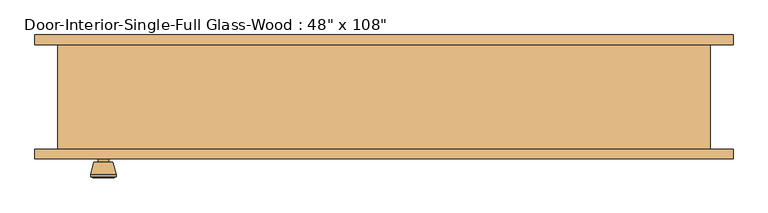
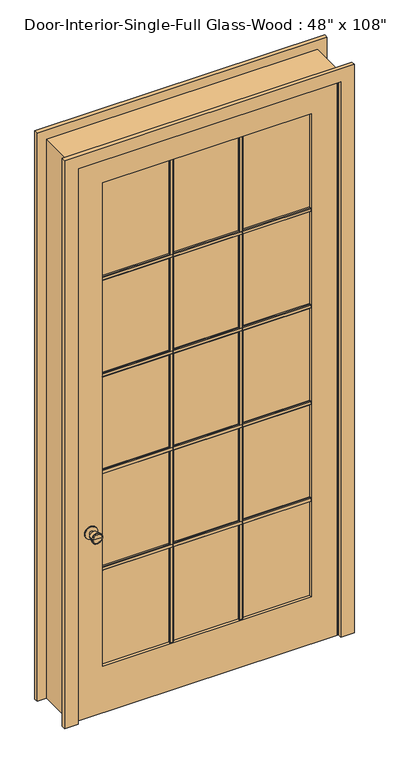
"""IFC4 building model written with IfcOpenShell, lengths in millimetres: door geometry."""

from ifc_helpers import new_model, si_unit, point, frame, frame_2d, origin, place, context, project, spatial, polyline, circle_curve, trimmed, segment, composite_curve, outline, extrude, faceted_brep, source, transform, mapped, element, save
from ifc_brep_helpers import plane_surface, cylinder_surface, revolved_surface, advanced_brep


def door_b9d6288b(model_context):
    return source(origin(), model_context, "Body", "SolidModel", [
        extrude(outline(polyline([(-84.455, 2155.19), (-84.455, 2136.14), (-90.805, 2136.14), (-93.98, 2139.315), (-93.98, 2152.015), (-90.805, 2155.19), (-84.455, 2155.19)])), frame((-488.95, 0.0, 0.0), z_axis=(1.0, 0.0, 0.0), x_axis=(0.0, 1.0, 0.0)), (0.0, 0.0, 1.0), 977.9),
        extrude(outline(polyline([(-84.455, 1676.7175), (-84.455, 1657.6675), (-90.805, 1657.6675), (-93.98, 1660.8425), (-93.98, 1673.5425), (-90.805, 1676.7175), (-84.455, 1676.7175)])), frame((-488.95, 0.0, 0.0), z_axis=(1.0, 0.0, 0.0), x_axis=(0.0, 1.0, 0.0)), (0.0, 0.0, 1.0), 977.9),
        extrude(outline(polyline([(-84.455, 1198.245), (-84.455, 1179.195), (-90.805, 1179.195), (-93.98, 1182.37), (-93.98, 1195.07), (-90.805, 1198.245), (-84.455, 1198.245)])), frame((-488.95, 0.0, 0.0), z_axis=(1.0, 0.0, 0.0), x_axis=(0.0, 1.0, 0.0)), (0.0, 0.0, 1.0), 977.9),
        extrude(outline(polyline([(-84.455, 719.7725), (-84.455, 700.7225), (-90.805, 700.7225), (-93.98, 703.8975), (-93.98, 716.5975), (-90.805, 719.7725), (-84.455, 719.7725)])), frame((-488.95, 0.0, 0.0), z_axis=(1.0, 0.0, 0.0), x_axis=(0.0, 1.0, 0.0)), (0.0, 0.0, 1.0), 977.9),
        extrude(outline(polyline([(153.4583333, -84.455), (172.5083333, -84.455), (172.5083333, -90.805), (169.3333333, -93.98), (156.6333333, -93.98), (153.4583333, -90.805), (153.4583333, -84.455)])), frame((0.0, 0.0, 231.775), z_axis=(0.0, 0.0, 1.0), x_axis=(1.0, 0.0, 0.0)), (0.0, 0.0, 1.0), 2392.3625),
        extrude(outline(polyline([(-172.5083333, -84.455), (-153.4583333, -84.455), (-153.4583333, -90.805), (-156.6333333, -93.98), (-169.3333333, -93.98), (-172.5083333, -90.805), (-172.5083333, -84.455)])), frame((0.0, 0.0, 231.775), z_axis=(0.0, 0.0, 1.0), x_axis=(1.0, 0.0, 0.0)), (0.0, 0.0, 1.0), 2392.3625),
        extrude(outline(polyline([(-77.47, 2155.19), (-71.12, 2155.19), (-67.945, 2152.015), (-67.945, 2139.315), (-71.12, 2136.14), (-77.47, 2136.14), (-77.47, 2155.19)])), frame((-488.95, 0.0, 0.0), z_axis=(1.0, 0.0, 0.0), x_axis=(0.0, 1.0, 0.0)), (0.0, 0.0, 1.0), 977.9),
        extrude(outline(polyline([(-77.47, 1676.7175), (-71.12, 1676.7175), (-67.945, 1673.5425), (-67.945, 1660.8425), (-71.12, 1657.6675), (-77.47, 1657.6675), (-77.47, 1676.7175)])), frame((-488.95, 0.0, 0.0), z_axis=(1.0, 0.0, 0.0), x_axis=(0.0, 1.0, 0.0)), (0.0, 0.0, 1.0), 977.9),
        extrude(outline(polyline([(-77.47, 1198.245), (-71.12, 1198.245), (-67.945, 1195.07), (-67.945, 1182.37), (-71.12, 1179.195), (-77.47, 1179.195), (-77.47, 1198.245)])), frame((-488.95, 0.0, 0.0), z_axis=(1.0, 0.0, 0.0), x_axis=(0.0, 1.0, 0.0)), (0.0, 0.0, 1.0), 977.9),
        extrude(outline(polyline([(-77.47, 719.7725), (-71.12, 719.7725), (-67.945, 716.5975), (-67.945, 703.8975), (-71.12, 700.7225), (-77.47, 700.7225), (-77.47, 719.7725)])), frame((-488.95, 0.0, 0.0), z_axis=(1.0, 0.0, 0.0), x_axis=(0.0, 1.0, 0.0)), (0.0, 0.0, 1.0), 977.9),
        extrude(outline(polyline([(153.4583333, -77.47), (153.4583333, -71.12), (156.6333333, -67.945), (169.3333333, -67.945), (172.5083333, -71.12), (172.5083333, -77.47), (153.4583333, -77.47)])), frame((0.0, 0.0, 231.775), z_axis=(0.0, 0.0, 1.0), x_axis=(1.0, 0.0, 0.0)), (0.0, 0.0, 1.0), 2392.3625),
        extrude(outline(polyline([(-172.5083333, -77.47), (-172.5083333, -71.12), (-169.3333333, -67.945), (-156.6333333, -67.945), (-153.4583333, -71.12), (-153.4583333, -77.47), (-172.5083333, -77.47)])), frame((0.0, 0.0, 231.775), z_axis=(0.0, 0.0, 1.0), x_axis=(1.0, 0.0, 0.0)), (0.0, 0.0, 1.0), 2392.3625),
        advanced_brep(
        [(-546.1, -57.5, 914.4), (-556.1, -57.5, 914.4), (-536.1, -57.5, 914.4), (-525.6241324, -8.5, 914.4), (-566.5758676, -8.5, 914.4), (-546.1, -8.5, 914.4), (-521.1, -10.3278681, 914.4), (-571.1, -10.3278681, 914.4), (-521.1, -13.7915463, 914.4), (-571.1, -13.7915463, 914.4), (-527.463764, -38.5, 914.4), (-564.736236, -38.5, 914.4), (-536.1, -38.5, 914.4), (-556.1, -38.5, 914.4)],
        [
            (0, 1),
            (1, 2, circle_curve(frame((-546.1, -57.5, 914.4), z_axis=(0.0, -1.0, 0.0), x_axis=(-1.0, 0.0, 0.0)), 10.0)),
            (2, 0),
            (2, 1, circle_curve(frame((-546.1, -57.5, 914.4), z_axis=(0.0, -1.0, 0.0), x_axis=(-1.0, 0.0, 0.0)), 10.0)),
            (3, 4, circle_curve(frame((-546.1, -8.5, 914.4), z_axis=(0.0, 1.0, 0.0), x_axis=(-1.0, 0.0, 0.0)), 20.4758676)),
            (4, 5),
            (5, 3),
            (4, 3, circle_curve(frame((-546.1, -8.5, 914.4), z_axis=(0.0, 1.0, 0.0), x_axis=(-1.0, 0.0, 0.0)), 20.4758676)),
            (6, 7, circle_curve(frame((-546.1, -10.3278681, 914.4), z_axis=(0.0, 1.0, 0.0), x_axis=(-1.0, 0.0, 0.0)), 25.0)),
            (7, 4),
            (3, 6),
            (7, 6, circle_curve(frame((-546.1, -10.3278681, 914.4), z_axis=(0.0, 1.0, 0.0), x_axis=(-1.0, 0.0, 0.0)), 25.0)),
            (8, 9, circle_curve(frame((-546.1, -13.7915463, 914.4), z_axis=(0.0, 1.0, 0.0), x_axis=(-1.0, 0.0, 0.0)), 25.0)),
            (9, 7),
            (6, 8),
            (9, 8, circle_curve(frame((-546.1, -13.7915463, 914.4), z_axis=(0.0, 1.0, 0.0), x_axis=(-1.0, 0.0, 0.0)), 25.0)),
            (10, 11, circle_curve(frame((-546.1, -38.5, 914.4), z_axis=(0.0, 1.0, 0.0), x_axis=(-1.0, 0.0, 0.0)), 18.636236)),
            (11, 9),
            (8, 10),
            (11, 10, circle_curve(frame((-546.1, -38.5, 914.4), z_axis=(0.0, 1.0, 0.0), x_axis=(-1.0, 0.0, 0.0)), 18.636236)),
            (12, 13, circle_curve(frame((-546.1, -38.5, 914.4), z_axis=(0.0, 1.0, 0.0), x_axis=(-1.0, 0.0, 0.0)), 10.0)),
            (13, 11),
            (10, 12),
            (13, 12, circle_curve(frame((-546.1, -38.5, 914.4), z_axis=(0.0, 1.0, 0.0), x_axis=(-1.0, 0.0, 0.0)), 10.0)),
            (1, 13),
            (12, 2),
        ],
        [
            plane_surface(frame((-546.1, -57.5, 914.4), z_axis=(0.0, -1.0, 0.0), x_axis=(-1.0, 0.0, 0.0))),
            plane_surface(frame((-546.1, -8.5, 914.4), z_axis=(0.0, 1.0, 0.0), x_axis=(-1.0, 0.0, 0.0))),
            revolved_surface(polyline([(-566.5758676, -8.5, 914.4), (-571.1, -10.3278681, 914.4)]), (-546.1, -57.5, 914.4), (0.0, -1.0, 0.0)),
            cylinder_surface(frame((-546.1, -57.5, 914.4), z_axis=(0.0, -1.0, 0.0), x_axis=(-1.0, 0.0, 0.0)), 25.0),
            revolved_surface(polyline([(-571.1, -13.7915463, 914.4), (-564.736236, -38.5, 914.4)]), (-546.1, -57.5, 914.4), (0.0, -1.0, 0.0)),
            plane_surface(frame((-546.1, -38.5, 914.4), z_axis=(0.0, -1.0, 0.0), x_axis=(-1.0, 0.0, 0.0))),
            cylinder_surface(frame((-546.1, -57.5, 914.4), z_axis=(0.0, -1.0, 0.0), x_axis=(-1.0, 0.0, 0.0)), 10.0),
        ],
        [
            (0, [[1, 2, 3]]),
            (0, [[-3, 4, -1]]),
            (1, [[5, 6, 7]]),
            (1, [[8, -7, -6]]),
            (2, [[9, 10, -5, 11]]),
            (2, [[12, -11, -8, -10]]),
            (3, [[13, 14, -9, 15]]),
            (3, [[16, -15, -12, -14]]),
            (4, [[17, 18, -13, 19]]),
            (4, [[20, -19, -16, -18]]),
            (5, [[21, 22, -17, 23]]),
            (5, [[24, -23, -20, -22]]),
            (6, [[-2, 25, -21, 26]]),
            (6, [[-4, -26, -24, -25]]),
        ],
    ),
        extrude(outline(composite_curve([segment(trimmed(circle_curve(frame_2d((914.4, -546.1)), 30.0), [point((914.4, -576.1))], [point((914.4, -516.1))], False, "CARTESIAN"), True, "CONTINUOUS"), segment(trimmed(circle_curve(frame_2d((914.4, -546.1)), 30.0), [point((914.4, -516.1))], [point((914.4, -576.1))], False, "CARTESIAN"), True, "CONTINUOUS")], self_intersect=False)), frame((0.0, -63.5, 0.0), z_axis=(0.0, 1.0, 0.0), x_axis=(0.0, 0.0, 1.0)), (0.0, 0.0, 1.0), 6.0),
        advanced_brep(
        [(-546.1, -104.425, 914.4), (-536.1, -104.425, 914.4), (-556.1, -104.425, 914.4), (-525.6241324, -153.425, 914.4), (-546.1, -153.425, 914.4), (-566.5758676, -153.425, 914.4), (-521.1, -151.5971319, 914.4), (-571.1, -151.5971319, 914.4), (-521.1, -148.1334537, 914.4), (-571.1, -148.1334537, 914.4), (-527.463764, -123.425, 914.4), (-564.736236, -123.425, 914.4), (-536.1, -123.425, 914.4), (-556.1, -123.425, 914.4)],
        [
            (0, 1),
            (1, 2, circle_curve(frame((-546.1, -104.425, 914.4), z_axis=(0.0, 1.0, 0.0), x_axis=(-1.0, 0.0, 0.0)), 10.0)),
            (2, 0),
            (2, 1, circle_curve(frame((-546.1, -104.425, 914.4), z_axis=(0.0, 1.0, 0.0), x_axis=(-1.0, 0.0, 0.0)), 10.0)),
            (3, 4),
            (4, 5),
            (5, 3, circle_curve(frame((-546.1, -153.425, 914.4), z_axis=(0.0, -1.0, 0.0), x_axis=(-1.0, 0.0, 0.0)), 20.4758676)),
            (3, 5, circle_curve(frame((-546.1, -153.425, 914.4), z_axis=(0.0, -1.0, 0.0), x_axis=(-1.0, 0.0, 0.0)), 20.4758676)),
            (6, 3),
            (5, 7),
            (7, 6, circle_curve(frame((-546.1, -151.5971319, 914.4), z_axis=(0.0, -1.0, 0.0), x_axis=(-1.0, 0.0, 0.0)), 25.0)),
            (6, 7, circle_curve(frame((-546.1, -151.5971319, 914.4), z_axis=(0.0, -1.0, 0.0), x_axis=(-1.0, 0.0, 0.0)), 25.0)),
            (8, 6),
            (7, 9),
            (9, 8, circle_curve(frame((-546.1, -148.1334537, 914.4), z_axis=(0.0, -1.0, 0.0), x_axis=(-1.0, 0.0, 0.0)), 25.0)),
            (8, 9, circle_curve(frame((-546.1, -148.1334537, 914.4), z_axis=(0.0, -1.0, 0.0), x_axis=(-1.0, 0.0, 0.0)), 25.0)),
            (10, 8),
            (9, 11),
            (11, 10, circle_curve(frame((-546.1, -123.425, 914.4), z_axis=(0.0, -1.0, 0.0), x_axis=(-1.0, 0.0, 0.0)), 18.636236)),
            (10, 11, circle_curve(frame((-546.1, -123.425, 914.4), z_axis=(0.0, -1.0, 0.0), x_axis=(-1.0, 0.0, 0.0)), 18.636236)),
            (12, 10),
            (11, 13),
            (13, 12, circle_curve(frame((-546.1, -123.425, 914.4), z_axis=(0.0, -1.0, 0.0), x_axis=(-1.0, 0.0, 0.0)), 10.0)),
            (12, 13, circle_curve(frame((-546.1, -123.425, 914.4), z_axis=(0.0, -1.0, 0.0), x_axis=(-1.0, 0.0, 0.0)), 10.0)),
            (1, 12),
            (13, 2),
        ],
        [
            plane_surface(frame((-546.1, -104.425, 914.4), z_axis=(0.0, 1.0, 0.0), x_axis=(-1.0, 0.0, 0.0))),
            plane_surface(frame((-546.1, -153.425, 914.4), z_axis=(0.0, -1.0, 0.0), x_axis=(-1.0, 0.0, 0.0))),
            revolved_surface(polyline([(-566.5758676, -153.425, 914.4), (-571.1, -151.5971319, 914.4)]), (-546.1, -104.425, 914.4), (0.0, 1.0, 0.0)),
            cylinder_surface(frame((-546.1, -104.425, 914.4), z_axis=(0.0, 1.0, 0.0), x_axis=(-1.0, 0.0, 0.0)), 25.0),
            revolved_surface(polyline([(-571.1, -148.1334537, 914.4), (-564.736236, -123.425, 914.4)]), (-546.1, -104.425, 914.4), (0.0, 1.0, 0.0)),
            plane_surface(frame((-546.1, -123.425, 914.4), z_axis=(0.0, 1.0, 0.0), x_axis=(-1.0, 0.0, 0.0))),
            cylinder_surface(frame((-546.1, -104.425, 914.4), z_axis=(0.0, 1.0, 0.0), x_axis=(-1.0, 0.0, 0.0)), 10.0),
        ],
        [
            (0, [[1, 2, 3]]),
            (0, [[-3, 4, -1]]),
            (1, [[5, 6, 7]]),
            (1, [[-6, -5, 8]]),
            (2, [[9, -7, 10, 11]]),
            (2, [[-10, -8, -9, 12]]),
            (3, [[13, -11, 14, 15]]),
            (3, [[-14, -12, -13, 16]]),
            (4, [[17, -15, 18, 19]]),
            (4, [[-18, -16, -17, 20]]),
            (5, [[21, -19, 22, 23]]),
            (5, [[-22, -20, -21, 24]]),
            (6, [[25, -23, 26, -2]]),
            (6, [[-26, -24, -25, -4]]),
        ],
    ),
        extrude(outline(composite_curve([segment(trimmed(circle_curve(frame_2d((914.4, -546.1)), 30.0), [point((914.4, -576.1))], [point((914.4, -516.1))], False, "CARTESIAN"), True, "CONTINUOUS"), segment(trimmed(circle_curve(frame_2d((914.4, -546.1)), 30.0), [point((914.4, -516.1))], [point((914.4, -576.1))], False, "CARTESIAN"), True, "CONTINUOUS")], self_intersect=False)), frame((0.0, -104.425, 0.0), z_axis=(0.0, 1.0, 0.0), x_axis=(0.0, 0.0, 1.0)), (0.0, 0.0, 1.0), 6.0),
        extrude(outline(polyline([(2743.2, -609.6), (0.0, -609.6), (0.0, 609.6), (2743.2, 609.6), (2743.2, -609.6)]), holes=[polyline([(2624.1375, -488.95), (2624.1375, 488.95), (231.775, 488.95), (231.775, -488.95), (2624.1375, -488.95)])]), frame((0.0, -98.425, 0.0), z_axis=(0.0, 1.0, 0.0), x_axis=(0.0, 0.0, 1.0)), (0.0, 0.0, 1.0), 34.925),
        faceted_brep([(635.0, -98.425, 0.0), (609.6, -98.425, 0.0), (609.6, -63.5, 0.0), (596.9, -63.5, 0.0), (596.9, -28.575, 0.0), (609.6, -28.575, 0.0), (609.6, 104.775, 0.0), (635.0, 104.775, 0.0), (635.0, 104.775, 2768.6), (635.0, -98.425, 2768.6), (609.6, 104.775, 2743.2), (-609.6, 104.775, 2743.2), (-609.6, 104.775, 0.0), (-635.0, 104.775, 0.0), (-635.0, 104.775, 2768.6), (609.6, -28.575, 2743.2), (596.9, -28.575, 2730.5), (-596.9, -28.575, 2730.5), (-596.9, -28.575, 0.0), (-609.6, -28.575, 0.0), (-609.6, -28.575, 2743.2), (596.9, -63.5, 2730.5), (609.6, -63.5, 2743.2), (-609.6, -63.5, 2743.2), (-609.6, -63.5, 0.0), (-596.9, -63.5, 0.0), (-596.9, -63.5, 2730.5), (609.6, -98.425, 2743.2), (-635.0, -98.425, 2768.6), (-635.0, -98.425, 0.0), (-609.6, -98.425, 0.0), (-609.6, -98.425, 2743.2)], [[[0, 1, 2, 3, 4, 5, 6, 7]], [[7, 8, 9, 0]], [[6, 10, 11, 12, 13, 14, 8, 7]], [[5, 15, 10, 6]], [[4, 16, 17, 18, 19, 20, 15, 5]], [[3, 21, 16, 4]], [[2, 22, 23, 24, 25, 26, 21, 3]], [[1, 27, 22, 2]], [[0, 9, 28, 29, 30, 31, 27, 1]], [[8, 14, 28, 9]], [[15, 20, 11, 10]], [[21, 26, 17, 16]], [[27, 31, 23, 22]], [[29, 13, 12, 19, 18, 25, 24, 30]], [[14, 13, 29, 28]], [[20, 19, 12, 11]], [[26, 25, 18, 17]], [[31, 30, 24, 23]]]),
        extrude(outline(polyline([(488.95, -77.47), (488.95, -84.455), (-488.95, -84.455), (-488.95, -77.47), (488.95, -77.47)])), frame((0.0, 0.0, 231.775), z_axis=(0.0, 0.0, 1.0), x_axis=(1.0, 0.0, 0.0)), (0.0, 0.0, 1.0), 2392.3625),
        extrude(outline(polyline([(0.0, 679.45), (2813.05, 679.45), (2813.05, -679.45), (0.0, -679.45), (0.0, -615.95), (2749.55, -615.95), (2749.55, 615.95), (0.0, 615.95), (0.0, 679.45)])), frame((0.0, 104.775, 0.0), z_axis=(0.0, 1.0, 0.0), x_axis=(0.0, 0.0, 1.0)), (0.0, 0.0, 1.0), 19.05),
        extrude(outline(polyline([(0.0, 679.45), (2813.05, 679.45), (2813.05, -679.45), (0.0, -679.45), (0.0, -615.95), (2749.55, -615.95), (2749.55, 615.95), (0.0, 615.95), (0.0, 679.45)])), frame((0.0, -117.475, 0.0), z_axis=(0.0, 1.0, 0.0), x_axis=(0.0, 0.0, 1.0)), (0.0, 0.0, 1.0), 19.05),
    ])


if __name__ == "__main__":
    model = new_model("IFC4")
    model_context = context("Model", 3, world=origin())
    ifc_project = project(units=[si_unit("LENGTHUNIT", "METRE", prefix="MILLI")], contexts=[model_context])
    site = spatial("IfcSite", under=ifc_project)
    building = spatial("IfcBuilding", under=site)
    placement = place(None, origin())
    door_shape = door_b9d6288b(model_context)
    element("IfcDoor", 1, ObjectType="Door-Interior-Single-Full Glass-Wood : 48\" x 108\"", at=placement, inside=building, context=model_context, shape_type="MappedRepresentation", body=[
        mapped(door_shape, transform((0.0, 0.0, 0.0), x_axis=(1.0, 0.0, 0.0), y_axis=(0.0, 1.0, 0.0), z_axis=(0.0, 0.0, 1.0))),
    ])
    save(model, "model.ifc")

# Revit data of these elements
# Type "Door-Interior-Single-Full Glass-Wood : 48\" x 108\""
#   Type Mark = "10"
#   Assembly Code = "C1020300"
#   Analytic Construction = "Wood frame with single clear glass"
#   Top Rail = 0' - 4 11/16"
#   Thickness = 0' - 1 3/8"
#   Thermal Resistance (R) = 1.0102 (h·ft²·°F)/BTU
#   Swing Angle [instance default] = 90.00°
#   Stiles = 0' - 4 3/4"
#   Rough Width = 4' - 2"
#   Rough Height = 9' - 1"
#   Height = 9' - 0"
#   Width = 4' - 0"
#   Heat Transfer Coefficient (U) = 0.9900 BTU/(h·ft²·°F)
#   Bottom Rail = 0' - 9 1/8"
#   Show Grill [instance default] = yes
#   Trim Material = Cherry
#   Panel Material = Brick, Common
#   Frame Material = Cherry
#   Door Handle Material = Aluminum
#   Visual Light Transmittance = 0
#   Solar Heat Gain Coefficient = 0
#   Wall Closure = (empty or 0)
#   Function = (empty or 0)
# Element 1 (IfcDoor, "Door-Interior-Single-Full Glass-Wood : 48\" x 108\"")
#   Materials on its faces: "Brick, Common", "Cherry", "Aluminum", "Glass"
# Materials
#   "Cherry": class "Wood", colour RGB 226 177 128, transparency 0, Description = "Prunus Serotina", Cost = 0
#   "Brick, Common": class "Masonry", colour RGB 170 98 104, transparency 0, Description = "Common brick", Cost = 0
#   "Aluminum": class "Metal", colour RGB 247 247 247, transparency 0, Description = "Aluminum 6061", Cost = 0
#   "Glass": class "Glass", colour RGB 0 128 192, transparency 0.75, Description = "Soda Lime Glass", Cost = 0
